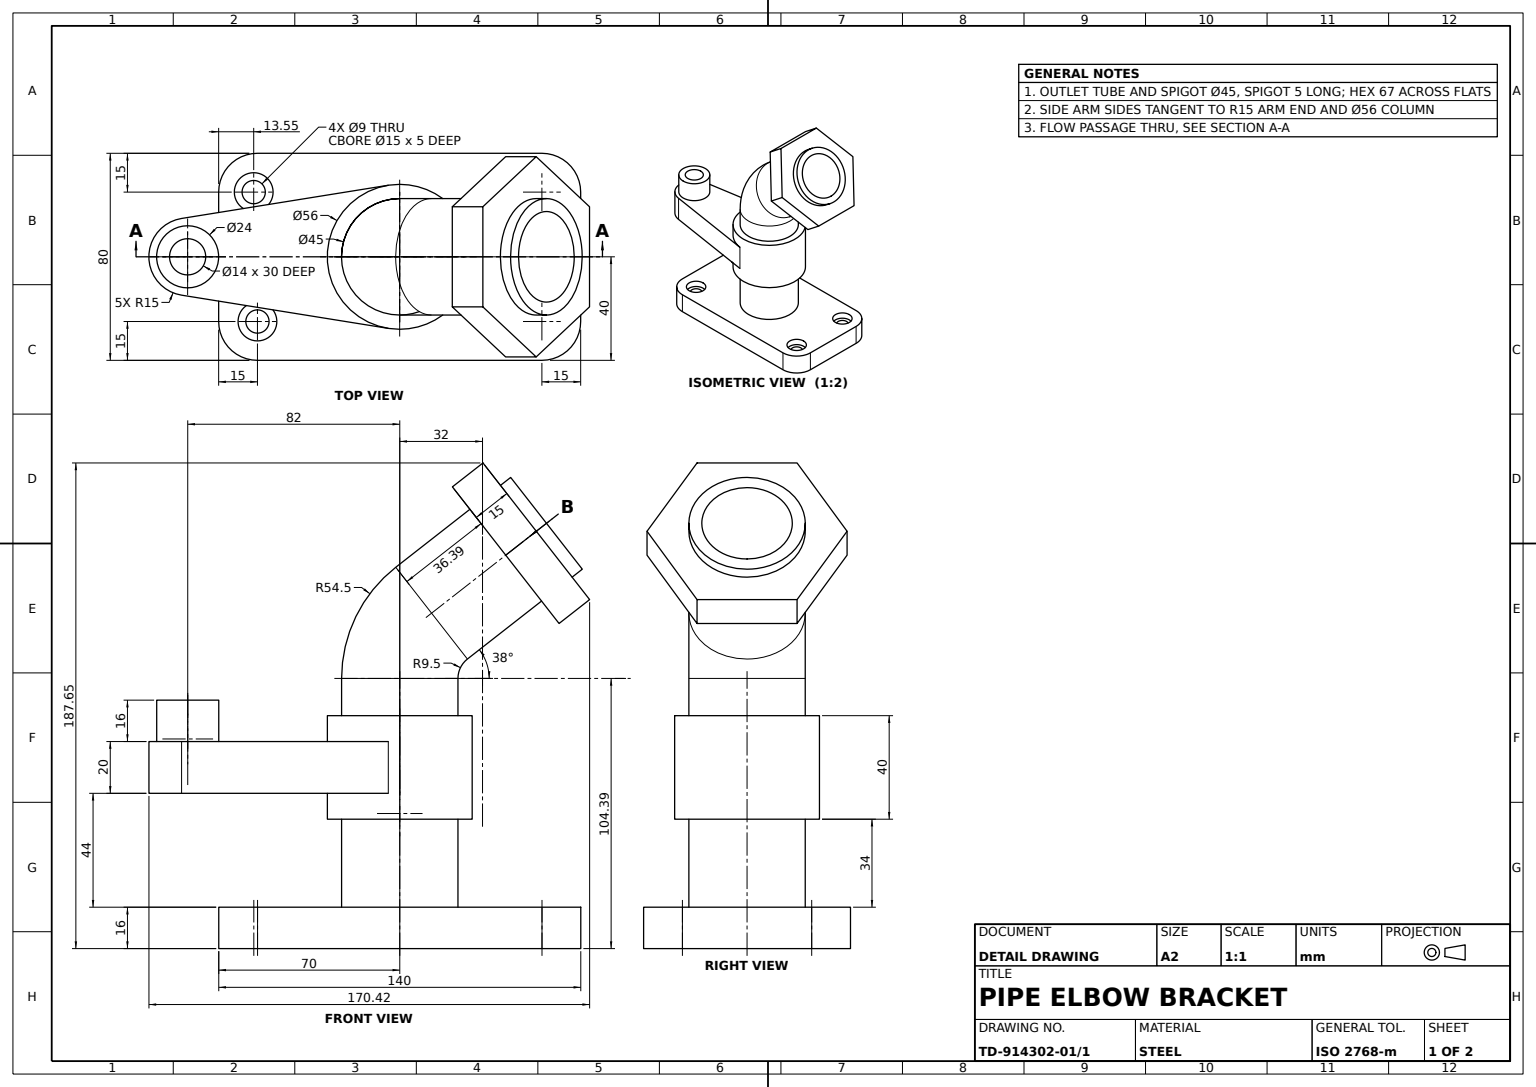
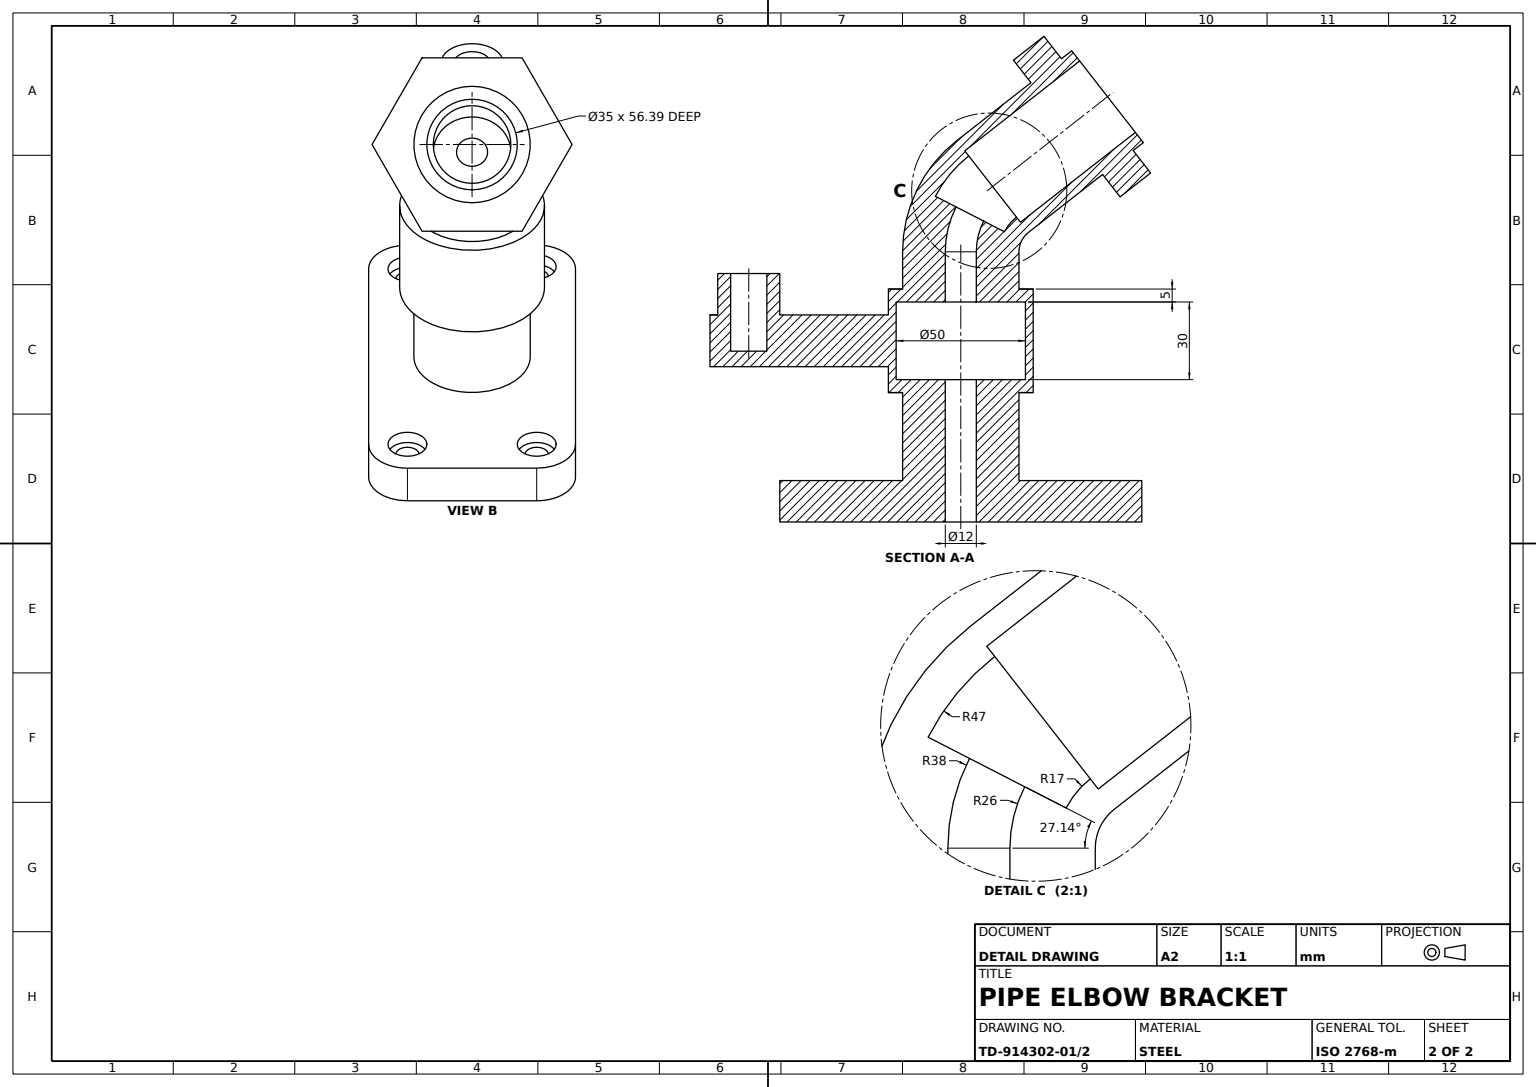
from build123d import *

# Parameters (mm, degrees)
BASE_PLATE_SKETCH_W                = 140
BASE_PLATE_SKETCH_H                = 80
BASE_PLATE_140X80X16_DEPTH         = 16
LOWER_COLUMN_SKETCH_R              = 22.5
LOWER_COLUMN_45_DEPTH              = 34
UPPER_COLUMN_SKETCH_R              = 28
UPPER_COLUMN_56_DEPTH              = 40
SIDE_ARM_DEPTH                     = 10
ELBOW_SWEEP_45_PROFILE_R           = 22.5
HEX_NUT_OUTLET_DEPTH               = 15
ARM_BOSS_SKETCH_R                  = 12
ARM_BOSS_24_DEPTH                  = 16
OUTLET_BORE_SKETCH_R               = 17.5
OUTLET_BORE_35_DEPTH               = 56.392557
ELBOW_PROFILE_CUT_PROFILE_R        = 15
FLOW_PASSAGE_12_PROFILE_R          = 6
COLUMN_GROOVE_SKETCH_W             = 25
COLUMN_GROOVE_SKETCH_H             = 30
ARM_BOSS_HOLE_SKETCH_R             = 7
ARM_BOSS_HOLE_14_DEPTH             = 30
BASE_PLATE_CORNER_FILLETS_R15_R    = 15
MOUNTING_HOLES_CBORE_9_D           = 9
MOUNTING_HOLES_CBORE_9_DEPTH       = 19.773719933
MOUNTING_HOLES_CBORE_9_CBORE_D     = 15
MOUNTING_HOLES_CBORE_9_CBORE_DEPTH = 5


with BuildPart() as part:
    # Base Plate Sketch → Base Plate 140x80x16 (new body)
    with BuildSketch(Plane(origin=(0, 0, 0), x_dir=(1, 0, 0), z_dir=(0, 1, 0))):
        Rectangle(BASE_PLATE_SKETCH_W, BASE_PLATE_SKETCH_H)
    extrude(amount=BASE_PLATE_140X80X16_DEPTH)

    # Lower Column Sketch → Lower Column _45 (add)
    with BuildSketch(Plane(origin=(0, 16, 0), x_dir=(1, 0, 0), z_dir=(0, 1, 0))):
        with Locations(Location((0, 0, 0), (0, 0, 270))):
            Circle(LOWER_COLUMN_SKETCH_R)
    extrude(amount=LOWER_COLUMN_45_DEPTH)

    # Upper Column Sketch → Upper Column _56 (add)
    with BuildSketch(Plane(origin=(0, 50, 0), x_dir=(1, 0, 0), z_dir=(0, 1, 0))):
        with Locations(Location((0, 0, 0), (0, 0, 270))):
            Circle(UPPER_COLUMN_SKETCH_R)
    extrude(amount=UPPER_COLUMN_56_DEPTH)

    # Side Arm Sketch → Side Arm (add, symmetric)
    with BuildSketch(Plane(origin=(0, 70, 0), x_dir=(1, 0, 0), z_dir=(0, 1, 0))):
        with BuildLine():
            Line((-84.37804878, 14.810296553), (-4.43902439, 27.6458869))
            ThreePointArc((-4.43902439, 27.6458869), (-28, 0), (-4.43902439, -27.6458869))
            Line((-4.43902439, -27.6458869), (-84.37804878, -14.810296553))
            ThreePointArc((-84.37804878, -14.810296553), (-97, 0), (-84.37804878, 14.810296553))
        make_face()
    extrude(amount=SIDE_ARM_DEPTH, both=True)

    # Elbow Sweep _45: sweep along a path in Elbow Path Sketch
    with BuildLine(Plane.XY) as elbow_sweep_45_path:
        Line((0, 0), (0, 104.392557166))
        ThreePointArc((0, 104.392557166), (3.238590518, 118.420433863), (12.29883279, 129.608901281))
        Line((12.29883279, 129.608901281), (56.73677426, 164.327626223))
    # Elbow Sweep _45 profile (on start of the path) → Elbow Sweep _45 (sweep)
    with BuildSketch(Plane.ZX):
        Circle(ELBOW_SWEEP_45_PROFILE_R)
    sweep(path=elbow_sweep_45_path.line)

    # Hex Nut Sketch → Hex Nut Outlet (add)
    with BuildSketch(Plane(origin=(111.014464068, 86.734005111, 0), x_dir=(0, 0, -1), z_dir=(0.7880107536067209, 0.6156614753256597, 0))):
        Polygon((-38.682468036, 94.561290433), (-19.341234018, 61.061290433), (19.341234018, 61.061290433), (38.682468036, 94.561290433), (19.341234018, 128.061290433), (-19.341234018, 128.061290433), align=None)
    extrude(amount=-HEX_NUT_OUTLET_DEPTH)

    # Arm Boss Sketch → Arm Boss _24 (add)
    with BuildSketch(Plane(origin=(0, 80, 0), x_dir=(1, 0, 0), z_dir=(0, 1, 0))):
        with Locations(Location((-82, 0, 0), (0, 0, 270))):
            Circle(ARM_BOSS_SKETCH_R)
    extrude(amount=ARM_BOSS_24_DEPTH)

    # Outlet Bore Sketch → Outlet Bore _35 (cut)
    with BuildSketch(Plane(origin=(114.954517836, 89.812312487, 0), x_dir=(0, 0, -1), z_dir=(0.7880107536067209, 0.6156614753256597, 0))):
        with Locations(Location((0, 94.561290433, 0), (0, 0, 90))):
            Circle(OUTLET_BORE_SKETCH_R)
    extrude(amount=-OUTLET_BORE_35_DEPTH, mode=Mode.SUBTRACT)

    # Elbow Profile Cut: sweep along a path in Elbow Profile Cut Sketch
    with BuildLine(Plane.XY) as elbow_profile_cut_path:
        Line((56.73677426, 164.327626223), (12.29883279, 129.608901281))
        ThreePointArc((12.29883279, 129.608901281), (7.332840345, 124.777140423), (3.523289487, 118.989712997))
    # Elbow Profile Cut profile (on start of the path) → Elbow Profile Cut (sweep, cut)
    with BuildSketch(Plane(origin=(56.73677426, 164.327626223, 0), x_dir=(0.6156614753256594, -0.7880107536067211, 0), z_dir=(-0.7880107536067211, -0.6156614753256594, 0))):
        Circle(ELBOW_PROFILE_CUT_PROFILE_R)
    sweep(path=elbow_profile_cut_path.line, mode=Mode.SUBTRACT)

    # Flow Passage _12: sweep along a path in Sketch5_4
    with BuildLine(Plane.XY) as flow_passage_12_path:
        Line((0, 0), (0, 104.392557166))
        ThreePointArc((0, 104.392557166), (3.238590518, 118.420433863), (12.29883279, 129.608901281))
        Line((12.29883279, 129.608901281), (56.73677426, 164.327626223))
    # Flow Passage _12 profile (on start of the path) → Flow Passage _12 (sweep, cut)
    with BuildSketch(Plane.ZX):
        Circle(FLOW_PASSAGE_12_PROFILE_R)
    sweep(path=flow_passage_12_path.line, mode=Mode.SUBTRACT)

    # Column Groove Sketch → Column Groove (revolve, cut)
    with BuildSketch(Plane.XY):
        with Locations((-12.5, 70)):
            Rectangle(COLUMN_GROOVE_SKETCH_W, COLUMN_GROOVE_SKETCH_H)
    revolve(axis=Axis((0, 55, 0), (0, 1, 0)), mode=Mode.SUBTRACT)

    # Arm Boss Hole Sketch → Arm Boss Hole _14 (cut)
    with BuildSketch(Plane(origin=(0, 96, 0), x_dir=(1, 0, 0), z_dir=(0, 1, 0))):
        with Locations(Location((-82, 0, 0), (0, 0, 270))):
            Circle(ARM_BOSS_HOLE_SKETCH_R)
    extrude(amount=-ARM_BOSS_HOLE_14_DEPTH, mode=Mode.SUBTRACT)

    # Base Plate Corner Fillets R15
    base_plate_corner_fillets_r15_edges = [part.edges().sort_by_distance(p)[0] for p in [
        (70, 8, 40),
        (-70, 8, 40),
        (-70, 8, -40),
        (70, 8, -40),
    ]]
    fillet(base_plate_corner_fillets_r15_edges, radius=BASE_PLATE_CORNER_FILLETS_R15_R)

    # Mounting Holes CBore _9
    with Locations(Plane(origin=(0, 16, 0), x_dir=(1, 0, 0), z_dir=(0, 1, 0))):
        with Locations((55, -25), (55, 25), (-56.445631344, 25), (-55, -25)):
            CounterBoreHole(MOUNTING_HOLES_CBORE_9_D / 2, MOUNTING_HOLES_CBORE_9_CBORE_D / 2, MOUNTING_HOLES_CBORE_9_CBORE_DEPTH, depth=MOUNTING_HOLES_CBORE_9_DEPTH)


solid = part.part
